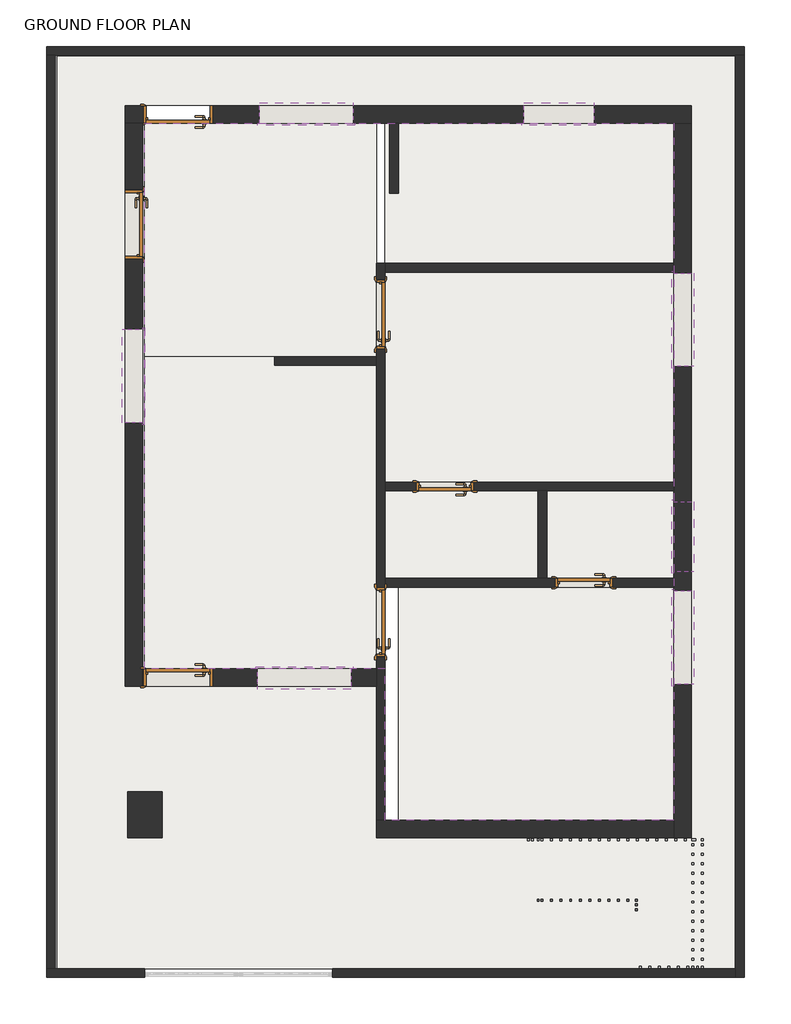
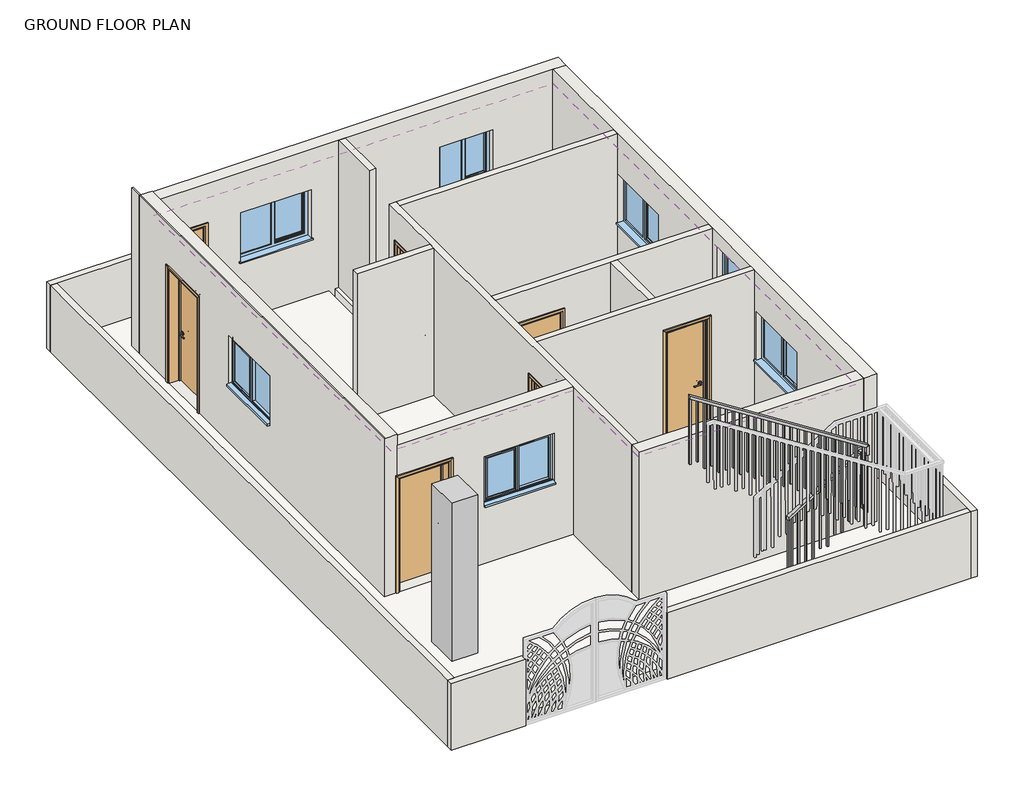
# One storey, part 1 of 23: 17 walls, 8 slabs, 7 doors, 7 windows, 1 column, 1 covering, 1 railing.
"""IFC4 building model written with IfcOpenShell, lengths in millimetres."""

from ifc_helpers import new_model, si_unit, frame, origin, place, context, project, spatial, polyline, outline, extrude, faceted_brep, transform, mapped, element, save
from components import columns_rectangular_450x600mm_2bb2af66, doors_intsgl_d1_d2de26da, doors_intsgl_d1_5aeab8eb, doors_intsgl_d1_91024936, doors_intsgl_d2_21b53886, doors_intsgl_d2_1f5f3f16, windows_dbl_plain_w1_9e0d93ab, windows_dbl_plain_w2_c69f14ef, windows_sgl_plain_v_28d0678b

model = new_model("IFC4")

# Units and contexts
model_context = context("Model", 3, world=origin())
ifc_project = project(units=[si_unit("LENGTHUNIT", "METRE", prefix="MILLI")], contexts=[model_context])

# Site, building, storey
site = spatial("IfcSite", under=ifc_project)
building = spatial("IfcBuilding", under=site)
storey = spatial("IfcBuildingStorey", under=building, Name="GROUND FLOOR PLAN", Elevation=487.68)

# Column
placement = place(None, origin())
columns_rectangular_450x600mm_shape = columns_rectangular_450x600mm_2bb2af66(model_context)
element("IfcColumn", 1, ObjectType="Columns_Rectangular : 450x600mm", at=placement, inside=storey, context=model_context, shape_type="MappedRepresentation", body=[
    mapped(columns_rectangular_450x600mm_shape, transform((-13810.4335145, -9915.2345894, 0.0), x_axis=(0.0, 1.0, 0.0), y_axis=(-1.0, 0.0, 0.0), z_axis=(0.0, 0.0, 1.0))),
])

# Covering
element("IfcCovering", 2, at=placement, inside=storey, context=model_context, shape_type="SweptSolid", body=[
    extrude(outline(polyline([(-6897.0620435, -885.5593981), (-6897.0620435, -9991.0521308), (-10668.9827978, -9991.0521308), (-10668.9827978, -8010.2345894), (-13810.6009005, -8010.2345894), (-13810.6009005, -885.5593981), (-6897.0620435, -885.5593981)])), frame((0.0, 0.0, 3078.48), z_axis=(0.0, 0.0, 1.0), x_axis=(1.0, 0.0, 0.0)), (0.0, 0.0, 1.0), 57.0),
])

# Doors
doors_intsgl_d1_shape = doors_intsgl_d1_d2de26da(model_context)
element("IfcDoor", 3, ObjectType="Doors_IntSgl : D1", at=placement, inside=storey, context=model_context, shape_type="MappedRepresentation", body=[
    mapped(doors_intsgl_d1_shape, transform((-10726.1327978, -7400.866169, 637.6416), x_axis=(0.0, 1.0, 0.0), y_axis=(-1.0, 0.0, 0.0), z_axis=(0.0, 0.0, 1.0))),
])
element("IfcDoor", 4, ObjectType="Doors_IntSgl : D1", at=placement, inside=storey, context=model_context, shape_type="MappedRepresentation", body=[
    mapped(doors_intsgl_d1_shape, transform((-10726.1327978, -3381.2262014, 637.6416), x_axis=(0.0, 1.0, 0.0), y_axis=(-1.0, 0.0, 0.0), z_axis=(0.0, 0.0, 1.0))),
])
doors_intsgl_d1_2_shape = doors_intsgl_d1_5aeab8eb(model_context)
element("IfcDoor", 5, ObjectType="Doors_IntSgl : D1", at=placement, inside=storey, context=model_context, shape_type="MappedRepresentation", body=[
    mapped(doors_intsgl_d1_2_shape, transform((-13373.8823015, -8124.5345894, 637.6416), x_axis=(-1.0, 0.0, 0.0), y_axis=(0.0, -1.0, 0.0), z_axis=(0.0, 0.0, 1.0))),
])
doors_intsgl_d1_3_shape = doors_intsgl_d1_91024936(model_context)
element("IfcDoor", 6, ObjectType="Doors_IntSgl : D1", at=placement, inside=storey, context=model_context, shape_type="MappedRepresentation", body=[
    mapped(doors_intsgl_d1_3_shape, transform((-13950.6420435, -2206.3593981, 637.6416), x_axis=(0.0, -1.0, 0.0), y_axis=(1.0, 0.0, 0.0), z_axis=(0.0, 0.0, 1.0))),
])
element("IfcDoor", 7, ObjectType="Doors_IntSgl : D1", at=placement, inside=storey, context=model_context, shape_type="MappedRepresentation", body=[
    mapped(doors_intsgl_d1_3_shape, transform((-13373.8823015, -771.2593981, 487.68), x_axis=(-1.0, 0.0, 0.0), y_axis=(0.0, -1.0, 0.0), z_axis=(0.0, 0.0, 1.0))),
])
doors_intsgl_d2_shape = doors_intsgl_d2_21b53886(model_context)
element("IfcDoor", 8, ObjectType="Doors_IntSgl : D2", at=placement, inside=storey, context=model_context, shape_type="MappedRepresentation", body=[
    mapped(doors_intsgl_d2_shape, transform((-9886.3340108, -5628.9784114, 637.6416), x_axis=(-1.0, 0.0, 0.0), y_axis=(0.0, -1.0, 0.0), z_axis=(0.0, 0.0, 1.0))),
])
doors_intsgl_d2_2_shape = doors_intsgl_d2_1f5f3f16(model_context)
element("IfcDoor", 9, ObjectType="Doors_IntSgl : D2", at=placement, inside=storey, context=model_context, shape_type="MappedRepresentation", body=[
    mapped(doors_intsgl_d2_2_shape, transform((-8070.4366309, -6886.516169, 637.6416), x_axis=(-1.0, 0.0, 0.0), y_axis=(0.0, -1.0, 0.0), z_axis=(0.0, 0.0, 1.0))),
])

# Railing
element("IfcRailing", 10, ObjectType="1100mm", at=placement, inside=storey, context=model_context, shape_type="SolidModel", body=[
    faceted_brep([(-8680.149573, -11007.9255223, 1912.8), (-8680.149573, -11007.9255223, 1853.4423995), (-8680.149573, -11057.9255223, 1853.4423995), (-8680.149573, -11057.9255223, 1912.8), (-7484.3306254, -11007.9255223, 2677.8717446), (-7434.3306254, -11007.9255223, 2650.5035914), (-7434.3306254, -11057.9255223, 2650.5035914), (-7484.3306254, -11057.9255223, 2677.8717446), (-7484.3306254, -11007.9255223, 2725.6), (-7434.3306254, -11007.9255223, 2675.6), (-7434.3306254, -11057.9255223, 2675.6), (-7484.3306254, -11057.9255223, 2725.6), (-7359.3306254, -11007.9255223, 2725.6), (-7359.3306254, -11007.9255223, 2675.6), (-7409.3306254, -11057.9255223, 2675.6), (-7409.3306254, -11057.9255223, 2725.6), (-7359.3306254, -11132.9255223, 2725.6), (-7359.3306254, -11132.9255223, 2675.6), (-7409.3306254, -11132.9255223, 2675.6), (-7409.3306254, -11132.9255223, 2725.6), (-7359.3306254, -11134.9255223, 2725.6), (-7409.3306254, -11134.9255223, 2725.6), (-7409.3306254, -11184.9255223, 2675.6), (-7359.3306254, -11184.9255223, 2675.6)], [[[0, 1, 2, 3]], [[1, 0, 4, 5]], [[2, 1, 5, 6]], [[3, 2, 6, 7]], [[0, 3, 7, 4]], [[5, 4, 8, 9]], [[6, 5, 9, 10]], [[7, 6, 10, 11]], [[4, 7, 11, 8]], [[9, 8, 12, 13]], [[10, 9, 13, 14]], [[11, 10, 14, 15]], [[8, 11, 15, 12]], [[13, 12, 16, 17]], [[14, 13, 17, 18]], [[15, 14, 18, 19]], [[12, 15, 19, 16]], [[20, 21, 22, 23]], [[17, 16, 20, 23]], [[18, 17, 23, 22]], [[19, 18, 22, 21]], [[16, 19, 21, 20]]]),
    faceted_brep([(-7359.3306254, -11134.9255223, 2725.6), (-7359.3306254, -11184.9255223, 2675.6), (-7409.3306254, -11184.9255223, 2675.6), (-7409.3306254, -11134.9255223, 2725.6), (-7359.3306254, -11134.9255223, 2855.9055527), (-7409.3306254, -11134.9255223, 2828.5415543), (-7409.3306254, -11184.9255223, 2828.5415543), (-7359.3306254, -11184.9255223, 2855.9055527)], [[[0, 1, 2, 3]], [[4, 5, 6, 7]], [[1, 0, 4, 7]], [[2, 1, 7, 6]], [[3, 2, 6, 5]], [[0, 3, 5, 4]]]),
    faceted_brep([(-7359.3306254, -11184.9255223, 2855.9055527), (-7409.3306254, -11184.9255223, 2828.5415543), (-7409.3306254, -11134.9255223, 2828.5415543), (-7359.3306254, -11134.9255223, 2855.9055527), (-10457.8773536, -11184.9255223, 4838.88), (-10457.8773536, -11134.9255223, 4838.88), (-10457.8773536, -11134.9255223, 4779.517542), (-10457.8773536, -11184.9255223, 4779.517542)], [[[0, 1, 2, 3]], [[4, 5, 6, 7]], [[1, 0, 4, 7]], [[2, 1, 7, 6]], [[3, 2, 6, 5]], [[0, 3, 5, 4]]]),
    extrude(outline(polyline([(3576.32, -10434.3306254), (4764.4483614, -10434.3306254), (4780.4475912, -10459.3306254), (3576.32, -10459.3306254), (3576.32, -10434.3306254)])), frame((0.0, -11172.4255223, 0.0), z_axis=(0.0, 1.0, 0.0), x_axis=(0.0, 0.0, 1.0)), (0.0, 0.0, 1.0), 25.0),
    extrude(outline(polyline([(3576.32, -10309.3306254), (4684.4522123, -10309.3306254), (4700.4514422, -10334.3306254), (3576.32, -10334.3306254), (3576.32, -10309.3306254)])), frame((0.0, -11172.4255223, 0.0), z_axis=(0.0, 1.0, 0.0), x_axis=(0.0, 0.0, 1.0)), (0.0, 0.0, 1.0), 25.0),
    extrude(outline(polyline([(3413.76, -10184.3306254), (4604.4560633, -10184.3306254), (4620.4552931, -10209.3306254), (3413.76, -10209.3306254), (3413.76, -10184.3306254)])), frame((0.0, -11172.4255223, 0.0), z_axis=(0.0, 1.0, 0.0), x_axis=(0.0, 0.0, 1.0)), (0.0, 0.0, 1.0), 25.0),
    extrude(outline(polyline([(3413.76, -10059.3306254), (4524.4599142, -10059.3306254), (4540.459144, -10084.3306254), (3413.76, -10084.3306254), (3413.76, -10059.3306254)])), frame((0.0, -11172.4255223, 0.0), z_axis=(0.0, 1.0, 0.0), x_axis=(0.0, 0.0, 1.0)), (0.0, 0.0, 1.0), 25.0),
    extrude(outline(polyline([(3251.2, -9934.3306254), (4444.4637652, -9934.3306254), (4460.462995, -9959.3306254), (3251.2, -9959.3306254), (3251.2, -9934.3306254)])), frame((0.0, -11172.4255223, 0.0), z_axis=(0.0, 1.0, 0.0), x_axis=(0.0, 0.0, 1.0)), (0.0, 0.0, 1.0), 25.0),
    extrude(outline(polyline([(3251.2, -9809.3306254), (4364.4676161, -9809.3306254), (4380.4668459, -9834.3306254), (3251.2, -9834.3306254), (3251.2, -9809.3306254)])), frame((0.0, -11172.4255223, 0.0), z_axis=(0.0, 1.0, 0.0), x_axis=(0.0, 0.0, 1.0)), (0.0, 0.0, 1.0), 25.0),
    extrude(outline(polyline([(3251.2, -9684.3306254), (4284.4714671, -9684.3306254), (4300.4706969, -9709.3306254), (3251.2, -9709.3306254), (3251.2, -9684.3306254)])), frame((0.0, -11172.4255223, 0.0), z_axis=(0.0, 1.0, 0.0), x_axis=(0.0, 0.0, 1.0)), (0.0, 0.0, 1.0), 25.0),
    extrude(outline(polyline([(3088.64, -9559.3306254), (4204.475318, -9559.3306254), (4220.4745478, -9584.3306254), (3088.64, -9584.3306254), (3088.64, -9559.3306254)])), frame((0.0, -11172.4255223, 0.0), z_axis=(0.0, 1.0, 0.0), x_axis=(0.0, 0.0, 1.0)), (0.0, 0.0, 1.0), 25.0),
    extrude(outline(polyline([(3088.64, -9434.3306254), (4124.479169, -9434.3306254), (4140.4783988, -9459.3306254), (3088.64, -9459.3306254), (3088.64, -9434.3306254)])), frame((0.0, -11172.4255223, 0.0), z_axis=(0.0, 1.0, 0.0), x_axis=(0.0, 0.0, 1.0)), (0.0, 0.0, 1.0), 25.0),
    extrude(outline(polyline([(2926.08, -9309.3306254), (4044.4830199, -9309.3306254), (4060.4822497, -9334.3306254), (2926.08, -9334.3306254), (2926.08, -9309.3306254)])), frame((0.0, -11172.4255223, 0.0), z_axis=(0.0, 1.0, 0.0), x_axis=(0.0, 0.0, 1.0)), (0.0, 0.0, 1.0), 25.0),
    extrude(outline(polyline([(2926.08, -9184.3306254), (3964.4868709, -9184.3306254), (3980.4861007, -9209.3306254), (2926.08, -9209.3306254), (2926.08, -9184.3306254)])), frame((0.0, -11172.4255223, 0.0), z_axis=(0.0, 1.0, 0.0), x_axis=(0.0, 0.0, 1.0)), (0.0, 0.0, 1.0), 25.0),
    extrude(outline(polyline([(2763.52, -9059.3306254), (3884.4907218, -9059.3306254), (3900.4899516, -9084.3306254), (2763.52, -9084.3306254), (2763.52, -9059.3306254)])), frame((0.0, -11172.4255223, 0.0), z_axis=(0.0, 1.0, 0.0), x_axis=(0.0, 0.0, 1.0)), (0.0, 0.0, 1.0), 25.0),
    extrude(outline(polyline([(2763.52, -8934.3306254), (3804.4945728, -8934.3306254), (3820.4938026, -8959.3306254), (2763.52, -8959.3306254), (2763.52, -8934.3306254)])), frame((0.0, -11172.4255223, 0.0), z_axis=(0.0, 1.0, 0.0), x_axis=(0.0, 0.0, 1.0)), (0.0, 0.0, 1.0), 25.0),
    extrude(outline(polyline([(2600.96, -8809.3306254), (3724.4984237, -8809.3306254), (3740.4976535, -8834.3306254), (2600.96, -8834.3306254), (2600.96, -8809.3306254)])), frame((0.0, -11172.4255223, 0.0), z_axis=(0.0, 1.0, 0.0), x_axis=(0.0, 0.0, 1.0)), (0.0, 0.0, 1.0), 25.0),
    extrude(outline(polyline([(2600.96, -8684.3306254), (3644.5022747, -8684.3306254), (3660.5015045, -8709.3306254), (2600.96, -8709.3306254), (2600.96, -8684.3306254)])), frame((0.0, -11172.4255223, 0.0), z_axis=(0.0, 1.0, 0.0), x_axis=(0.0, 0.0, 1.0)), (0.0, 0.0, 1.0), 25.0),
    extrude(outline(polyline([(2438.4, -8559.3306254), (3564.5061256, -8559.3306254), (3580.5053554, -8584.3306254), (2438.4, -8584.3306254), (2438.4, -8559.3306254)])), frame((0.0, -11172.4255223, 0.0), z_axis=(0.0, 1.0, 0.0), x_axis=(0.0, 0.0, 1.0)), (0.0, 0.0, 1.0), 25.0),
    extrude(outline(polyline([(2438.4, -8434.3306254), (3484.5099766, -8434.3306254), (3500.5092064, -8459.3306254), (2438.4, -8459.3306254), (2438.4, -8434.3306254)])), frame((0.0, -11172.4255223, 0.0), z_axis=(0.0, 1.0, 0.0), x_axis=(0.0, 0.0, 1.0)), (0.0, 0.0, 1.0), 25.0),
    extrude(outline(polyline([(2275.84, -8309.3306254), (3404.5138275, -8309.3306254), (3420.5130573, -8334.3306254), (2275.84, -8334.3306254), (2275.84, -8309.3306254)])), frame((0.0, -11172.4255223, 0.0), z_axis=(0.0, 1.0, 0.0), x_axis=(0.0, 0.0, 1.0)), (0.0, 0.0, 1.0), 25.0),
    extrude(outline(polyline([(2275.84, -8184.3306254), (3324.5176785, -8184.3306254), (3340.5169083, -8209.3306254), (2275.84, -8209.3306254), (2275.84, -8184.3306254)])), frame((0.0, -11172.4255223, 0.0), z_axis=(0.0, 1.0, 0.0), x_axis=(0.0, 0.0, 1.0)), (0.0, 0.0, 1.0), 25.0),
    extrude(outline(polyline([(2113.28, -8059.3306254), (3244.5215294, -8059.3306254), (3260.5207592, -8084.3306254), (2113.28, -8084.3306254), (2113.28, -8059.3306254)])), frame((0.0, -11172.4255223, 0.0), z_axis=(0.0, 1.0, 0.0), x_axis=(0.0, 0.0, 1.0)), (0.0, 0.0, 1.0), 25.0),
    extrude(outline(polyline([(2113.28, -7934.3306254), (3164.5253804, -7934.3306254), (3180.5246102, -7959.3306254), (2113.28, -7959.3306254), (2113.28, -7934.3306254)])), frame((0.0, -11172.4255223, 0.0), z_axis=(0.0, 1.0, 0.0), x_axis=(0.0, 0.0, 1.0)), (0.0, 0.0, 1.0), 25.0),
    extrude(outline(polyline([(1950.72, -7809.3306254), (3084.5292313, -7809.3306254), (3100.5284611, -7834.3306254), (1950.72, -7834.3306254), (1950.72, -7809.3306254)])), frame((0.0, -11172.4255223, 0.0), z_axis=(0.0, 1.0, 0.0), x_axis=(0.0, 0.0, 1.0)), (0.0, 0.0, 1.0), 25.0),
    extrude(outline(polyline([(1950.72, -7684.3306254), (3004.5330823, -7684.3306254), (3020.5323121, -7709.3306254), (1950.72, -7709.3306254), (1950.72, -7684.3306254)])), frame((0.0, -11172.4255223, 0.0), z_axis=(0.0, 1.0, 0.0), x_axis=(0.0, 0.0, 1.0)), (0.0, 0.0, 1.0), 25.0),
    extrude(outline(polyline([(1788.16, -7559.3306254), (2924.5369332, -7559.3306254), (2940.536163, -7584.3306254), (1788.16, -7584.3306254), (1788.16, -7559.3306254)])), frame((0.0, -11172.4255223, 0.0), z_axis=(0.0, 1.0, 0.0), x_axis=(0.0, 0.0, 1.0)), (0.0, 0.0, 1.0), 25.0),
    extrude(outline(polyline([(1788.16, -7434.3306254), (2844.5407841, -7434.3306254), (2860.540014, -7459.3306254), (1788.16, -7459.3306254), (1788.16, -7434.3306254)])), frame((0.0, -11172.4255223, 0.0), z_axis=(0.0, 1.0, 0.0), x_axis=(0.0, 0.0, 1.0)), (0.0, 0.0, 1.0), 25.0),
    extrude(outline(polyline([(-7396.8306254, -11082.9255223), (-7371.8306254, -11082.9255223), (-7371.8306254, -11107.9255223), (-7396.8306254, -11107.9255223), (-7396.8306254, -11082.9255223)])), frame((0.0, 0.0, 1625.6), z_axis=(0.0, 0.0, 1.0), x_axis=(1.0, 0.0, 0.0)), (0.0, 0.0, 1.0), 1050.0),
    extrude(outline(polyline([(2605.1944115, -7505.149573), (1463.04, -7505.149573), (1463.04, -7480.149573), (2621.1891352, -7480.149573), (2605.1944115, -7505.149573)])), frame((0.0, -11045.4255223, 0.0), z_axis=(0.0, 1.0, 0.0), x_axis=(0.0, 0.0, 1.0)), (0.0, 0.0, 1.0), 25.0),
    extrude(outline(polyline([(2525.2207932, -7630.149573), (1463.04, -7630.149573), (1463.04, -7605.149573), (2541.2155169, -7605.149573), (2525.2207932, -7630.149573)])), frame((0.0, -11045.4255223, 0.0), z_axis=(0.0, 1.0, 0.0), x_axis=(0.0, 0.0, 1.0)), (0.0, 0.0, 1.0), 25.0),
    extrude(outline(polyline([(2445.2471749, -7755.149573), (1300.48, -7755.149573), (1300.48, -7730.149573), (2461.2418986, -7730.149573), (2445.2471749, -7755.149573)])), frame((0.0, -11045.4255223, 0.0), z_axis=(0.0, 1.0, 0.0), x_axis=(0.0, 0.0, 1.0)), (0.0, 0.0, 1.0), 25.0),
    extrude(outline(polyline([(2365.2735566, -7880.149573), (1300.48, -7880.149573), (1300.48, -7855.149573), (2381.2682803, -7855.149573), (2365.2735566, -7880.149573)])), frame((0.0, -11045.4255223, 0.0), z_axis=(0.0, 1.0, 0.0), x_axis=(0.0, 0.0, 1.0)), (0.0, 0.0, 1.0), 25.0),
    extrude(outline(polyline([(2285.2999383, -8005.149573), (1137.92, -8005.149573), (1137.92, -7980.149573), (2301.294662, -7980.149573), (2285.2999383, -8005.149573)])), frame((0.0, -11045.4255223, 0.0), z_axis=(0.0, 1.0, 0.0), x_axis=(0.0, 0.0, 1.0)), (0.0, 0.0, 1.0), 25.0),
    extrude(outline(polyline([(2205.32632, -8130.149573), (1137.92, -8130.149573), (1137.92, -8105.149573), (2221.3210437, -8105.149573), (2205.32632, -8130.149573)])), frame((0.0, -11045.4255223, 0.0), z_axis=(0.0, 1.0, 0.0), x_axis=(0.0, 0.0, 1.0)), (0.0, 0.0, 1.0), 25.0),
    extrude(outline(polyline([(2125.3527017, -8255.149573), (975.36, -8255.149573), (975.36, -8230.149573), (2141.3474254, -8230.149573), (2125.3527017, -8255.149573)])), frame((0.0, -11045.4255223, 0.0), z_axis=(0.0, 1.0, 0.0), x_axis=(0.0, 0.0, 1.0)), (0.0, 0.0, 1.0), 25.0),
    extrude(outline(polyline([(2045.3790834, -8380.149573), (975.36, -8380.149573), (975.36, -8355.149573), (2061.3738071, -8355.149573), (2045.3790834, -8380.149573)])), frame((0.0, -11045.4255223, 0.0), z_axis=(0.0, 1.0, 0.0), x_axis=(0.0, 0.0, 1.0)), (0.0, 0.0, 1.0), 25.0),
    extrude(outline(polyline([(1965.4054651, -8505.149573), (812.8, -8505.149573), (812.8, -8480.149573), (1981.4001888, -8480.149573), (1965.4054651, -8505.149573)])), frame((0.0, -11045.4255223, 0.0), z_axis=(0.0, 1.0, 0.0), x_axis=(0.0, 0.0, 1.0)), (0.0, 0.0, 1.0), 25.0),
    extrude(outline(polyline([(1885.4318468, -8630.149573), (812.8, -8630.149573), (812.8, -8605.149573), (1901.4265705, -8605.149573), (1885.4318468, -8630.149573)])), frame((0.0, -11045.4255223, 0.0), z_axis=(0.0, 1.0, 0.0), x_axis=(0.0, 0.0, 1.0)), (0.0, 0.0, 1.0), 25.0),
    extrude(outline(polyline([(-7396.8306254, -11147.4255223), (-7371.8306254, -11147.4255223), (-7371.8306254, -11172.4255223), (-7396.8306254, -11172.4255223), (-7396.8306254, -11147.4255223)])), frame((0.0, 0.0, 1625.6), z_axis=(0.0, 0.0, 1.0), x_axis=(1.0, 0.0, 0.0)), (0.0, 0.0, 1.0), 1050.0),
    extrude(outline(polyline([(-7396.8306254, -11045.4255223), (-7396.8306254, -11020.4255223), (-7371.8306254, -11020.4255223), (-7371.8306254, -11045.4255223), (-7396.8306254, -11045.4255223)])), frame((0.0, 0.0, 1625.6), z_axis=(0.0, 0.0, 1.0), x_axis=(1.0, 0.0, 0.0)), (0.0, 0.0, 1.0), 1050.0),
    extrude(outline(polyline([(3576.32, -10432.8773536), (4763.5183122, -10432.8773536), (4779.517542, -10457.8773536), (3576.32, -10457.8773536), (3576.32, -10432.8773536)])), frame((0.0, -11172.4255223, 0.0), z_axis=(0.0, 1.0, 0.0), x_axis=(0.0, 0.0, 1.0)), (0.0, 0.0, 1.0), 25.0),
    extrude(outline(polyline([(1853.4423995, -8680.149573), (812.8, -8680.149573), (812.8, -8655.149573), (1869.4371231, -8655.149573), (1853.4423995, -8680.149573)])), frame((0.0, -11045.4255223, 0.0), z_axis=(0.0, 1.0, 0.0), x_axis=(0.0, 0.0, 1.0)), (0.0, 0.0, 1.0), 25.0),
])

# Slabs
element("IfcSlab", 11, ObjectType="BATHROOM FLOORING", at=placement, inside=storey, context=model_context, shape_type="SweptSolid", body=[
    extrude(outline(polyline([(-8667.3366309, -5686.1284114), (-8667.3366309, -6829.366169), (-10668.9827978, -6829.366169), (-10668.9827978, -5686.1284114), (-8667.3366309, -5686.1284114)])), frame((0.0, 0.0, 487.68), z_axis=(0.0, 0.0, 1.0), x_axis=(1.0, 0.0, 0.0)), (0.0, 0.0, 1.0), 149.9616),
])
element("IfcSlab", 12, ObjectType="BATHROOM FLOORING", at=placement, inside=storey, context=model_context, shape_type="SweptSolid", body=[
    extrude(outline(polyline([(-6724.371003, -5686.0601635), (-6724.371003, -6829.366169), (-8553.0366309, -6829.366169), (-8553.0366309, -5686.0601635), (-6724.371003, -5686.0601635)])), frame((0.0, 0.0, 487.68), z_axis=(0.0, 0.0, 1.0), x_axis=(1.0, 0.0, 0.0)), (0.0, 0.0, 1.0), 149.9616),
])
element("IfcSlab", 13, ObjectType="BED ROOM FLOORING", at=placement, inside=storey, context=model_context, shape_type="SweptSolid", body=[
    extrude(outline(polyline([(-6724.371003, -2828.9136626), (-6724.371003, -5571.8284114), (-10668.9827978, -5571.8284114), (-10668.9827978, -2828.9136626), (-6724.371003, -2828.9136626)])), frame((0.0, 0.0, 487.68), z_axis=(0.0, 0.0, 1.0), x_axis=(1.0, 0.0, 0.0)), (0.0, 0.0, 1.0), 149.9616),
])
element("IfcSlab", 14, ObjectType="BED ROOM FLOORING", at=placement, inside=storey, context=model_context, shape_type="SweptSolid", body=[
    extrude(outline(polyline([(-6698.6395131, -6943.5979211), (-6698.6395131, -9991.1886267), (-10495.9340108, -9991.1886267), (-10495.9340108, -6943.5979211), (-6698.6395131, -6943.5979211)])), frame((0.0, 0.0, 487.68), z_axis=(0.0, 0.0, 1.0), x_axis=(1.0, 0.0, 0.0)), (0.0, 0.0, 1.0), 149.9616),
])
element("IfcSlab", 15, ObjectType="DINING FLOORING", at=placement, inside=storey, context=model_context, shape_type="SweptSolid", body=[
    extrude(outline(polyline([(-10783.2827978, -885.9480347), (-10783.2827978, -3933.5387403), (-13810.6009005, -3933.5387403), (-13810.6009005, -885.9480347), (-10783.2827978, -885.9480347)])), frame((0.0, 0.0, 487.68), z_axis=(0.0, 0.0, 1.0), x_axis=(1.0, 0.0, 0.0)), (0.0, 0.0, 1.0), 149.9616),
])
element("IfcSlab", 16, ObjectType="HALL FLOORING", at=placement, inside=storey, context=model_context, shape_type="SweptSolid", body=[
    extrude(outline(polyline([(-10783.2827978, -3933.5387403), (-10783.2827978, -8010.2345894), (-13810.6009005, -8010.2345894), (-13810.6009005, -3933.5387403), (-10783.2827978, -3933.5387403)])), frame((0.0, 0.0, 487.68), z_axis=(0.0, 0.0, 1.0), x_axis=(1.0, 0.0, 0.0)), (0.0, 0.0, 1.0), 149.9616),
])
element("IfcSlab", 17, ObjectType="KITCHEN FLOOR", at=placement, inside=storey, context=model_context, shape_type="SweptSolid", body=[
    extrude(outline(polyline([(-6724.371003, -885.9480347), (-6724.371003, -2714.6136626), (-10668.9827978, -2714.6136626), (-10668.9827978, -885.9480347), (-6724.371003, -885.9480347)])), frame((0.0, 0.0, 487.68), z_axis=(0.0, 0.0, 1.0), x_axis=(1.0, 0.0, 0.0)), (0.0, 0.0, 1.0), 149.9616),
])
element("IfcSlab", 18, ObjectType="OUTER FLOORING", at=placement, inside=storey, context=model_context, shape_type="Brep", body=[
    faceted_brep([(-6089.3420435, -9.6873231, 487.68), (-6089.3420435, -11928.1928911, 487.68), (-14953.3817735, -11928.1928911, 487.68), (-14953.3817735, -9.6873231, 487.68), (-6668.4620435, -656.9593981, 487.68), (-12916.6823015, -656.9593981, 487.68), (-13831.0823015, -656.9593981, 487.68), (-14064.9420435, -656.9593981, 487.68), (-14064.9420435, -885.5593981, 487.68), (-14064.9420435, -8238.8345894, 487.68), (-13836.3420435, -8238.8345894, 487.68), (-10783.2827978, -8238.8345894, 487.68), (-10783.2827978, -9991.0521308, 487.68), (-10783.2827978, -10219.6521308, 487.68), (-6897.0620435, -10219.6521308, 487.68), (-6668.4620435, -10219.6521308, 487.68), (-6668.4620435, -885.5593981, 487.68), (-6089.3420435, -9.6873231, 637.6416), (-14953.3817735, -9.6873231, 637.6416), (-14953.3817735, -11928.1928911, 637.6416), (-6089.3420435, -11928.1928911, 637.6416), (-6668.4620435, -656.9593981, 637.6416), (-6668.4620435, -10219.6521308, 637.6416), (-10783.2827978, -10219.6521308, 637.6416), (-10783.2827978, -8238.8345894, 637.6416), (-12916.6823015, -8238.8345894, 637.6416), (-13831.0823015, -8238.8345894, 637.6416), (-14064.9420435, -8238.8345894, 637.6416), (-14064.9420435, -2663.5593981, 637.6416), (-14064.9420435, -1749.1593981, 637.6416), (-14064.9420435, -656.9593981, 637.6416)], [[[0, 1, 2, 3], [4, 5, 6, 7, 8, 9, 10, 11, 12, 13, 14, 15, 16]], [[17, 18, 19, 20], [21, 22, 23, 24, 25, 26, 27, 28, 29, 30]], [[1, 0, 17, 20]], [[2, 1, 20, 19]], [[3, 2, 19, 18]], [[0, 3, 18, 17]], [[7, 6, 5, 4, 21, 30]], [[9, 8, 7, 30, 29, 28, 27]], [[11, 10, 9, 27, 26, 25, 24]], [[13, 12, 11, 24, 23]], [[15, 14, 13, 23, 22]], [[4, 16, 15, 22, 21]]]),
])

# Walls
element("IfcWall", 19, at=placement, inside=storey, context=model_context, shape_type="Brep", body=[
    faceted_brep([(-15093.6420435, 3.4571089, 487.68), (-14979.3420435, 3.4571089, 487.68), (-6089.3420435, 3.4571089, 487.68), (-5975.0420435, 3.4571089, 487.68), (-5975.0420435, 3.4571089, 1706.88), (-6089.3420435, 3.4571089, 1706.88), (-14979.3420435, 3.4571089, 1706.88), (-15093.6420435, 3.4571089, 1706.88), (-15093.6420435, 117.7571089, 487.68), (-15093.6420435, 117.7571089, 1706.88), (-5975.0420435, 117.7571089, 1706.88), (-5975.0420435, 117.7571089, 487.68)], [[[0, 1, 2, 3, 4, 5, 6, 7]], [[8, 9, 10, 11]], [[3, 2, 1, 0, 8, 11]], [[7, 6, 5, 4, 10, 9]], [[4, 3, 11, 10]], [[0, 7, 9, 8]]]),
])
element("IfcWall", 20, at=placement, inside=storey, context=model_context, shape_type="Brep", body=[
    faceted_brep([(-6089.3420435, 3.4571089, 487.68), (-6089.3420435, -11928.1928911, 487.68), (-6089.3420435, -12042.4928911, 487.68), (-6089.3420435, -12042.4928911, 1706.88), (-6089.3420435, -11928.1928911, 1706.88), (-6089.3420435, 3.4571089, 1706.88), (-5975.0420435, 3.4571089, 487.68), (-5975.0420435, 3.4571089, 1706.88), (-5975.0420435, -12042.4928911, 1706.88), (-5975.0420435, -12042.4928911, 487.68)], [[[0, 1, 2, 3, 4, 5]], [[6, 7, 8, 9]], [[2, 1, 0, 6, 9]], [[5, 4, 3, 8, 7]], [[0, 5, 7, 6]], [[3, 2, 9, 8]]]),
])
element("IfcWall", 21, at=placement, inside=storey, context=model_context, shape_type="SweptSolid", body=[
    extrude(outline(polyline([(-11356.3590108, -11928.1928911), (-6089.3420435, -11928.1928911), (-6089.3420435, -12042.4928911), (-11356.3590108, -12042.4928911), (-11356.3590108, -11928.1928911)])), frame((0.0, 0.0, 487.68), z_axis=(0.0, 0.0, 1.0), x_axis=(1.0, 0.0, 0.0)), (0.0, 0.0, 1.0), 1219.2),
])
element("IfcWall", 22, at=placement, inside=storey, context=model_context, shape_type="SweptSolid", body=[
    extrude(outline(polyline([(-14979.3420435, 3.4571089), (-14979.3420435, -11928.1928911), (-15093.6420435, -11928.1928911), (-15093.6420435, 3.4571089), (-14979.3420435, 3.4571089)])), frame((0.0, 0.0, 487.68), z_axis=(0.0, 0.0, 1.0), x_axis=(1.0, 0.0, 0.0)), (0.0, 0.0, 1.0), 1219.2),
])
element("IfcWall", 23, at=placement, inside=storey, context=model_context, shape_type="Brep", body=[
    faceted_brep([(-13810.4335145, -11928.1928911, 487.68), (-14979.3420435, -11928.1928911, 487.68), (-15093.6420435, -11928.1928911, 487.68), (-15093.6420435, -11928.1928911, 1706.88), (-14979.3420435, -11928.1928911, 1706.88), (-13810.4335145, -11928.1928911, 1706.88), (-13810.4335145, -12042.4928911, 487.68), (-13810.4335145, -12042.4928911, 1706.88), (-15093.6420435, -12042.4928911, 1706.88), (-15093.6420435, -12042.4928911, 487.68)], [[[0, 1, 2, 3, 4, 5]], [[6, 7, 8, 9]], [[2, 1, 0, 6, 9]], [[5, 4, 3, 8, 7]], [[0, 5, 7, 6]], [[3, 2, 9, 8]]]),
])
element("IfcWall", 24, ObjectType="EXT WALL", at=placement, inside=storey, context=model_context, shape_type="Brep", body=[
    faceted_brep([(-14064.9420435, -885.5593981, 487.68), (-13836.3420435, -885.5593981, 487.68), (-13831.0823015, -885.5593981, 487.68), (-13831.0823015, -885.5593981, 2597.68), (-12916.6823015, -885.5593981, 2597.68), (-12916.6823015, -885.5593981, 487.68), (-6897.0620435, -885.5593981, 487.68), (-6668.4620435, -885.5593981, 487.68), (-6668.4620435, -885.5593981, 637.6416), (-6668.4620435, -885.5593981, 3335.7312), (-6897.0620435, -885.5593981, 3335.7312), (-14039.0335145, -885.5593981, 3335.7312), (-14039.0335145, -885.5593981, 3535.68), (-14064.9420435, -885.5593981, 3535.68), (-14064.9420435, -885.5593981, 637.6416), (-12307.0823015, -885.5593981, 1687.68), (-12307.0823015, -885.5593981, 2597.68), (-11087.8823015, -885.5593981, 2597.68), (-11087.8823015, -885.5593981, 1687.68), (-8852.8620435, -885.5593981, 1687.68), (-8852.8620435, -885.5593981, 2597.68), (-7938.4620435, -885.5593981, 2597.68), (-7938.4620435, -885.5593981, 1687.68), (-13831.0823015, -656.9593981, 487.68), (-14064.9420435, -656.9593981, 487.68), (-14064.9420435, -656.9593981, 637.6416), (-14064.9420435, -656.9593981, 3535.68), (-14039.0335145, -656.9593981, 3535.68), (-14039.0335145, -656.9593981, 3335.7312), (-6668.4620435, -656.9593981, 3335.7312), (-6668.4620435, -656.9593981, 637.6416), (-6668.4620435, -656.9593981, 487.68), (-12916.6823015, -656.9593981, 487.68), (-12916.6823015, -656.9593981, 637.6416), (-12916.6823015, -656.9593981, 2597.68), (-13831.0823015, -656.9593981, 2597.68), (-13831.0823015, -656.9593981, 637.6416), (-12307.0823015, -656.9593981, 2597.68), (-12307.0823015, -656.9593981, 1687.68), (-11087.8823015, -656.9593981, 1687.68), (-11087.8823015, -656.9593981, 2597.68), (-8852.8620435, -656.9593981, 2597.68), (-8852.8620435, -656.9593981, 1687.68), (-7938.4620435, -656.9593981, 1687.68), (-7938.4620435, -656.9593981, 2597.68)], [[[0, 1, 2, 3, 4, 5, 6, 7, 8, 9, 10, 11, 12, 13, 14], [15, 16, 17, 18], [19, 20, 21, 22]], [[23, 24, 25, 26, 27, 28, 29, 30, 31, 32, 33, 34, 35, 36], [37, 38, 39, 40], [41, 42, 43, 44]], [[31, 7, 6, 5, 32]], [[0, 24, 23, 2, 1]], [[7, 31, 30, 29, 9, 8]], [[24, 0, 14, 13, 26, 25]], [[35, 3, 2, 23, 36]], [[3, 35, 34, 4]], [[4, 34, 33, 32, 5]], [[38, 37, 16, 15]], [[39, 38, 15, 18]], [[40, 39, 18, 17]], [[37, 40, 17, 16]], [[42, 41, 20, 19]], [[43, 42, 19, 22]], [[44, 43, 22, 21]], [[41, 44, 21, 20]], [[28, 11, 10, 9, 29]], [[11, 28, 27, 12]], [[13, 12, 27, 26]]]),
])
element("IfcWall", 25, ObjectType="EXT WALL", at=placement, inside=storey, context=model_context, shape_type="Brep", body=[
    faceted_brep([(-6897.0620435, -885.5593981, 487.68), (-6897.0620435, -5571.8284114, 487.68), (-6897.0620435, -5686.1284114, 487.68), (-6897.0620435, -9991.0521308, 487.68), (-6897.0620435, -10219.6521308, 487.68), (-6897.0620435, -10219.6521308, 637.6416), (-6897.0620435, -10219.6521308, 3335.7312), (-6897.0620435, -9991.0521308, 3335.7312), (-6897.0620435, -6943.666169, 3335.7312), (-6897.0620435, -6829.366169, 3335.7312), (-6897.0620435, -5686.1284114, 3335.7312), (-6897.0620435, -5571.8284114, 3335.7312), (-6897.0620435, -885.5593981, 3335.7312), (-6897.0620435, -6993.8521308, 1687.68), (-6897.0620435, -6993.8521308, 2597.68), (-6897.0620435, -8213.0521308, 2597.68), (-6897.0620435, -8213.0521308, 1687.68), (-6897.0620435, -2841.3593981, 1687.68), (-6897.0620435, -2841.3593981, 2597.68), (-6897.0620435, -4060.5593981, 2597.68), (-6897.0620435, -4060.5593981, 1687.68), (-6897.0620435, -5825.4521308, 2164.08), (-6897.0620435, -5825.4521308, 3074.08), (-6897.0620435, -6739.8521308, 3074.08), (-6897.0620435, -6739.8521308, 2164.08), (-6668.4620435, -10219.6521308, 487.68), (-6668.4620435, -885.5593981, 487.68), (-6668.4620435, -885.5593981, 637.6416), (-6668.4620435, -885.5593981, 3335.7312), (-6668.4620435, -10219.6521308, 3335.7312), (-6668.4620435, -10219.6521308, 637.6416), (-6668.4620435, -6993.8521308, 2597.68), (-6668.4620435, -6993.8521308, 1687.68), (-6668.4620435, -8213.0521308, 1687.68), (-6668.4620435, -8213.0521308, 2597.68), (-6668.4620435, -2841.3593981, 2597.68), (-6668.4620435, -2841.3593981, 1687.68), (-6668.4620435, -4060.5593981, 1687.68), (-6668.4620435, -4060.5593981, 2597.68), (-6668.4620435, -5825.4521308, 3074.08), (-6668.4620435, -5825.4521308, 2164.08), (-6668.4620435, -6739.8521308, 2164.08), (-6668.4620435, -6739.8521308, 3074.08)], [[[0, 1, 2, 3, 4, 5, 6, 7, 8, 9, 10, 11, 12], [13, 14, 15, 16], [17, 18, 19, 20], [21, 22, 23, 24]], [[25, 26, 27, 28, 29, 30], [31, 32, 33, 34], [35, 36, 37, 38], [39, 40, 41, 42]], [[4, 3, 2, 1, 0, 26, 25]], [[26, 0, 12, 28, 27]], [[4, 25, 30, 29, 6, 5]], [[32, 31, 14, 13]], [[33, 32, 13, 16]], [[34, 33, 16, 15]], [[31, 34, 15, 14]], [[36, 35, 18, 17]], [[37, 36, 17, 20]], [[38, 37, 20, 19]], [[35, 38, 19, 18]], [[40, 39, 22, 21]], [[41, 40, 21, 24]], [[42, 41, 24, 23]], [[39, 42, 23, 22]], [[12, 11, 10, 9, 8, 7, 6, 29, 28]]]),
])
element("IfcWall", 26, ObjectType="EXT WALL", at=placement, inside=storey, context=model_context, shape_type="Brep", body=[
    faceted_brep([(-6897.0620435, -9991.0521308, 487.68), (-10668.9827978, -9991.0521308, 487.68), (-10783.2827978, -9991.0521308, 487.68), (-10783.2827978, -9991.0521308, 637.6416), (-10783.2827978, -9991.0521308, 3335.7312), (-10668.9827978, -9991.0521308, 3335.7312), (-6897.0620435, -9991.0521308, 3335.7312), (-10783.2827978, -10219.6521308, 487.68), (-6897.0620435, -10219.6521308, 487.68), (-6897.0620435, -10219.6521308, 637.6416), (-6897.0620435, -10219.6521308, 3335.7312), (-10783.2827978, -10219.6521308, 3335.7312), (-10783.2827978, -10219.6521308, 637.6416)], [[[0, 1, 2, 3, 4, 5, 6]], [[7, 8, 9, 10, 11, 12]], [[2, 1, 0, 8, 7]], [[8, 0, 6, 10, 9]], [[2, 7, 12, 11, 4, 3]], [[6, 5, 4, 11, 10]]]),
])
element("IfcWall", 27, ObjectType="EXT WALL", at=placement, inside=storey, context=model_context, shape_type="Brep", body=[
    faceted_brep([(-14064.9420435, -885.5593981, 487.68), (-14064.9420435, -8238.8345894, 487.68), (-14064.9420435, -8238.8345894, 637.6416), (-14064.9420435, -8238.8345894, 3535.68), (-14064.9420435, -885.5593981, 3535.68), (-14064.9420435, -885.5593981, 637.6416), (-14064.9420435, -2663.5593981, 2747.6416), (-14064.9420435, -2663.5593981, 637.6416), (-14064.9420435, -1749.1593981, 637.6416), (-14064.9420435, -1749.1593981, 2747.6416), (-14064.9420435, -4797.1593981, 2597.68), (-14064.9420435, -4797.1593981, 1687.68), (-14064.9420435, -3577.9593981, 1687.68), (-14064.9420435, -3577.9593981, 2597.68), (-13836.3420435, -8238.8345894, 487.68), (-13836.3420435, -8010.2345894, 487.68), (-13836.3420435, -885.5593981, 487.68), (-13836.3420435, -885.5593981, 3535.68), (-13836.3420435, -8238.8345894, 3535.68), (-13836.3420435, -8238.8345894, 3335.7312), (-13836.3420435, -8238.8345894, 637.6416), (-13836.3420435, -2663.5593981, 637.6416), (-13836.3420435, -2663.5593981, 2747.6416), (-13836.3420435, -1749.1593981, 2747.6416), (-13836.3420435, -1749.1593981, 637.6416), (-13836.3420435, -4797.1593981, 1687.68), (-13836.3420435, -4797.1593981, 2597.68), (-13836.3420435, -3577.9593981, 2597.68), (-13836.3420435, -3577.9593981, 1687.68), (-14039.0335145, -885.5593981, 3535.68), (-14039.0335145, -8238.8345894, 3535.68)], [[[0, 1, 2, 3, 4, 5], [6, 7, 8, 9], [10, 11, 12, 13]], [[14, 15, 16, 17, 18, 19, 20], [21, 22, 23, 24], [25, 26, 27, 28]], [[1, 0, 16, 15, 14]], [[17, 16, 0, 5, 4, 29]], [[1, 14, 20, 19, 18, 30, 3, 2]], [[7, 6, 22, 21]], [[6, 9, 23, 22]], [[9, 8, 24, 23]], [[8, 7, 21, 24]], [[11, 10, 26, 25]], [[12, 11, 25, 28]], [[13, 12, 28, 27]], [[10, 13, 27, 26]], [[18, 17, 29, 30]], [[4, 3, 30, 29]]]),
])
element("IfcWall", 28, ObjectType="EXT WALL", at=placement, inside=storey, context=model_context, shape_type="Brep", body=[
    faceted_brep([(-13836.3420435, -8238.8345894, 487.68), (-10783.2827978, -8238.8345894, 487.68), (-10783.2827978, -8238.8345894, 637.6416), (-10783.2827978, -8238.8345894, 3335.7312), (-13836.3420435, -8238.8345894, 3335.7312), (-13836.3420435, -8238.8345894, 637.6416), (-13831.0823015, -8238.8345894, 637.6416), (-13831.0823015, -8238.8345894, 2747.6416), (-12916.6823015, -8238.8345894, 2747.6416), (-12916.6823015, -8238.8345894, 637.6416), (-11113.4827978, -8238.8345894, 2597.68), (-11113.4827978, -8238.8345894, 1687.68), (-12332.6827978, -8238.8345894, 1687.68), (-12332.6827978, -8238.8345894, 2597.68), (-10783.2827978, -8010.2345894, 487.68), (-13836.3420435, -8010.2345894, 487.68), (-13836.3420435, -8010.2345894, 3335.7312), (-10783.2827978, -8010.2345894, 3335.7312), (-13831.0823015, -8010.2345894, 2747.6416), (-13831.0823015, -8010.2345894, 637.6416), (-12916.6823015, -8010.2345894, 637.6416), (-12916.6823015, -8010.2345894, 2747.6416), (-11113.4827978, -8010.2345894, 1687.68), (-11113.4827978, -8010.2345894, 2597.68), (-12332.6827978, -8010.2345894, 2597.68), (-12332.6827978, -8010.2345894, 1687.68)], [[[0, 1, 2, 3, 4, 5], [6, 7, 8, 9], [10, 11, 12, 13]], [[14, 15, 16, 17], [18, 19, 20, 21], [22, 23, 24, 25]], [[1, 0, 15, 14]], [[15, 0, 5, 4, 16]], [[1, 14, 17, 3, 2]], [[18, 7, 6, 19]], [[7, 18, 21, 8]], [[8, 21, 20, 9]], [[19, 6, 9, 20]], [[11, 10, 23, 22]], [[12, 11, 22, 25]], [[13, 12, 25, 24]], [[10, 13, 24, 23]], [[4, 3, 17, 16]]]),
])
element("IfcWall", 29, ObjectType="INT WALL", at=placement, inside=storey, context=model_context, shape_type="SweptSolid", body=[
    extrude(outline(polyline([(-10610.2340108, -1800.3480347), (-10610.2340108, -885.9480347), (-10495.9340108, -885.9480347), (-10495.9340108, -1800.3480347), (-10610.2340108, -1800.3480347)])), frame((0.0, 0.0, 487.68), z_axis=(0.0, 0.0, 1.0), x_axis=(1.0, 0.0, 0.0)), (0.0, 0.0, 1.0), 2848.0512),
])
element("IfcWall", 30, ObjectType="INT WALL", at=placement, inside=storey, context=model_context, shape_type="SweptSolid", body=[
    extrude(outline(polyline([(-10668.9827978, -2714.6136626), (-6897.41979, -2714.6136626), (-6897.41979, -2828.9136626), (-10668.9827978, -2828.9136626), (-10668.9827978, -2714.6136626)])), frame((0.0, 0.0, 487.68), z_axis=(0.0, 0.0, 1.0), x_axis=(1.0, 0.0, 0.0)), (0.0, 0.0, 1.0), 2848.0512),
])
element("IfcWall", 31, ObjectType="INT WALL", at=placement, inside=storey, context=model_context, shape_type="Brep", body=[
    faceted_brep([(-10668.9827978, -5686.1284114, 487.68), (-8667.3366309, -5686.1284114, 487.68), (-8553.0366309, -5686.1284114, 487.68), (-6897.0620435, -5686.1284114, 487.68), (-6897.0620435, -5686.1284114, 3335.7312), (-8553.0366309, -5686.1284114, 3335.7312), (-8667.3366309, -5686.1284114, 3335.7312), (-10668.9827978, -5686.1284114, 3335.7312), (-10267.3340108, -5686.1284114, 637.6416), (-10267.3340108, -5686.1284114, 2747.6416), (-9505.3340108, -5686.1284114, 2747.6416), (-9505.3340108, -5686.1284114, 637.6416), (-6897.0620435, -5571.8284114, 487.68), (-10668.9827978, -5571.8284114, 487.68), (-10668.9827978, -5571.8284114, 3335.7312), (-6897.0620435, -5571.8284114, 3335.7312), (-10267.3340108, -5571.8284114, 2747.6416), (-10267.3340108, -5571.8284114, 637.6416), (-9505.3340108, -5571.8284114, 637.6416), (-9505.3340108, -5571.8284114, 2747.6416)], [[[0, 1, 2, 3, 4, 5, 6, 7], [8, 9, 10, 11]], [[12, 13, 14, 15], [16, 17, 18, 19]], [[3, 2, 1, 0, 13, 12]], [[13, 0, 7, 14]], [[8, 17, 16, 9]], [[9, 16, 19, 10]], [[18, 11, 10, 19]], [[17, 8, 11, 18]], [[7, 6, 5, 4, 15, 14]], [[3, 12, 15, 4]]]),
])
element("IfcWall", 32, ObjectType="INT WALL", at=placement, inside=storey, context=model_context, shape_type="Brep", body=[
    faceted_brep([(-10668.9827978, -6943.666169, 491.0136234), (-6897.0620435, -6943.666169, 491.0136234), (-6897.0620435, -6943.666169, 3335.7312), (-10668.9827978, -6943.666169, 3335.7312), (-10668.9827978, -6943.666169, 2747.6416), (-10668.9827978, -6943.666169, 637.6416), (-8451.4366309, -6943.666169, 637.6416), (-8451.4366309, -6943.666169, 2747.6416), (-7689.4366309, -6943.666169, 2747.6416), (-7689.4366309, -6943.666169, 637.6416), (-6897.0620435, -6829.366169, 491.0136234), (-10668.9827978, -6829.366169, 491.0136234), (-10668.9827978, -6829.366169, 3335.7312), (-8667.3366309, -6829.366169, 3335.7312), (-8553.0366309, -6829.366169, 3335.7312), (-6897.0620435, -6829.366169, 3335.7312), (-8451.4366309, -6829.366169, 2747.6416), (-8451.4366309, -6829.366169, 637.6416), (-7689.4366309, -6829.366169, 637.6416), (-7689.4366309, -6829.366169, 2747.6416)], [[[0, 1, 2, 3, 4, 5], [6, 7, 8, 9]], [[10, 11, 12, 13, 14, 15], [16, 17, 18, 19]], [[1, 0, 11, 10]], [[11, 0, 5, 4, 3, 12]], [[6, 17, 16, 7]], [[7, 16, 19, 8]], [[18, 9, 8, 19]], [[17, 6, 9, 18]], [[3, 2, 15, 14, 13, 12]], [[1, 10, 15, 2]]]),
])
element("IfcWall", 33, ObjectType="INT WALL", at=placement, inside=storey, context=model_context, shape_type="SweptSolid", body=[
    extrude(outline(polyline([(-8667.3366309, -6829.366169), (-8667.3366309, -5686.1284114), (-8553.0366309, -5686.1284114), (-8553.0366309, -6829.366169), (-8667.3366309, -6829.366169)])), frame((0.0, 0.0, 487.68), z_axis=(0.0, 0.0, 1.0), x_axis=(1.0, 0.0, 0.0)), (0.0, 0.0, 1.0), 2848.0512),
])
element("IfcWall", 34, ObjectType="INT WALL", at=placement, inside=storey, context=model_context, shape_type="SweptSolid", body=[
    extrude(outline(polyline([(-10783.2827978, -4047.8387403), (-12112.7859221, -4047.8387403), (-12112.7859221, -3933.5387403), (-10783.2827978, -3933.5387403), (-10783.2827978, -4047.8387403)])), frame((0.0, 0.0, 487.68), z_axis=(0.0, 0.0, 1.0), x_axis=(1.0, 0.0, 0.0)), (0.0, 0.0, 1.0), 2848.0512),
])
element("IfcWall", 35, ObjectType="INT WALL", at=placement, inside=storey, context=model_context, shape_type="Brep", body=[
    faceted_brep([(-10783.2827978, -9991.0521308, 3335.7312), (-10783.2827978, -8238.8345894, 3335.7312), (-10783.2827978, -8010.2345894, 3335.7312), (-10783.2827978, -4047.8387403, 3335.7312), (-10783.2827978, -3933.5387403, 3335.7312), (-10783.2827978, -2714.6136626, 3335.7312), (-10783.2827978, -2714.6136626, 487.68), (-10783.2827978, -3933.5387403, 487.68), (-10783.2827978, -4047.8387403, 487.68), (-10783.2827978, -8010.2345894, 487.68), (-10783.2827978, -8238.8345894, 487.68), (-10783.2827978, -9991.0521308, 487.68), (-10783.2827978, -9991.0521308, 637.6416), (-10783.2827978, -7858.066169, 637.6416), (-10783.2827978, -6943.666169, 637.6416), (-10783.2827978, -6943.666169, 2747.6416), (-10783.2827978, -7858.066169, 2747.6416), (-10783.2827978, -3838.4262014, 637.6416), (-10783.2827978, -2924.0262014, 637.6416), (-10783.2827978, -2924.0262014, 2747.6416), (-10783.2827978, -3838.4262014, 2747.6416), (-10668.9827978, -9991.0521308, 487.68), (-10668.9827978, -5686.1284114, 487.68), (-10668.9827978, -5571.8284114, 487.68), (-10668.9827978, -2828.9136626, 487.68), (-10668.9827978, -2714.6136626, 487.68), (-10668.9827978, -2714.6136626, 3335.7312), (-10668.9827978, -2828.9136626, 3335.7312), (-10668.9827978, -5571.8284114, 3335.7312), (-10668.9827978, -5686.1284114, 3335.7312), (-10668.9827978, -6829.366169, 3335.7312), (-10668.9827978, -6943.666169, 3335.7312), (-10668.9827978, -9991.0521308, 3335.7312), (-10668.9827978, -6943.666169, 637.6416), (-10668.9827978, -7858.066169, 637.6416), (-10668.9827978, -7858.066169, 2747.6416), (-10668.9827978, -6943.666169, 2747.6416), (-10668.9827978, -2924.0262014, 637.6416), (-10668.9827978, -3838.4262014, 637.6416), (-10668.9827978, -3838.4262014, 2747.6416), (-10668.9827978, -2924.0262014, 2747.6416)], [[[0, 1, 2, 3, 4, 5, 6, 7, 8, 9, 10, 11, 12], [13, 14, 15, 16], [17, 18, 19, 20]], [[21, 22, 23, 24, 25, 26, 27, 28, 29, 30, 31, 32], [33, 34, 35, 36], [37, 38, 39, 40]], [[25, 24, 23, 22, 21, 11, 10, 9, 8, 7, 6]], [[11, 21, 32, 0, 12]], [[14, 13, 34, 33]], [[13, 16, 35, 34]], [[16, 15, 36, 35]], [[15, 14, 33, 36]], [[18, 17, 38, 37]], [[17, 20, 39, 38]], [[20, 19, 40, 39]], [[19, 18, 37, 40]], [[5, 4, 3, 2, 1, 0, 32, 31, 30, 29, 28, 27, 26]], [[25, 6, 5, 26]]]),
])

# Windows
windows_dbl_plain_w1_shape = windows_dbl_plain_w1_9e0d93ab(model_context)
element("IfcWindow", 36, ObjectType="Windows_Dbl_Plain : W1", at=placement, inside=storey, context=model_context, shape_type="MappedRepresentation", body=[
    mapped(windows_dbl_plain_w1_shape, transform((-6791.2186113, -7888.4521308, 487.68), x_axis=(0.0, -1.0, 0.0), y_axis=(1.0, 0.0, 0.0), z_axis=(0.0, 0.0, 1.0))),
])
element("IfcWindow", 37, ObjectType="Windows_Dbl_Plain : W1", at=placement, inside=storey, context=model_context, shape_type="MappedRepresentation", body=[
    mapped(windows_dbl_plain_w1_shape, transform((-6791.2186113, -3735.9593981, 487.68), x_axis=(0.0, -1.0, 0.0), y_axis=(1.0, 0.0, 0.0), z_axis=(0.0, 0.0, 1.0))),
])
element("IfcWindow", 38, ObjectType="Windows_Dbl_Plain : W1", at=placement, inside=storey, context=model_context, shape_type="MappedRepresentation", body=[
    mapped(windows_dbl_plain_w1_shape, transform((-11412.4823015, -779.7159659, 487.68), x_axis=(1.0, 0.0, 0.0), y_axis=(0.0, 1.0, 0.0), z_axis=(0.0, 0.0, 1.0))),
])
element("IfcWindow", 39, ObjectType="Windows_Dbl_Plain : W1", at=placement, inside=storey, context=model_context, shape_type="MappedRepresentation", body=[
    mapped(windows_dbl_plain_w1_shape, transform((-13942.1854757, -3902.5593981, 487.68), x_axis=(0.0, 1.0, 0.0), y_axis=(-1.0, 0.0, 0.0), z_axis=(0.0, 0.0, 1.0))),
])
element("IfcWindow", 40, ObjectType="Windows_Dbl_Plain : W1", at=placement, inside=storey, context=model_context, shape_type="MappedRepresentation", body=[
    mapped(windows_dbl_plain_w1_shape, transform((-12008.0827978, -8116.0780216, 487.68), x_axis=(-1.0, 0.0, 0.0), y_axis=(0.0, -1.0, 0.0), z_axis=(0.0, 0.0, 1.0))),
])
windows_dbl_plain_w2_shape = windows_dbl_plain_w2_c69f14ef(model_context)
element("IfcWindow", 41, ObjectType="Windows_Dbl_Plain : W2", at=placement, inside=storey, context=model_context, shape_type="MappedRepresentation", body=[
    mapped(windows_dbl_plain_w2_shape, transform((-8110.6620435, -779.7159659, 487.68), x_axis=(1.0, 0.0, 0.0), y_axis=(0.0, 1.0, 0.0), z_axis=(0.0, 0.0, 1.0))),
])
windows_sgl_plain_v_shape = windows_sgl_plain_v_28d0678b(model_context)
element("IfcWindow", 42, ObjectType="Windows_Sgl_Plain : V", at=placement, inside=storey, context=model_context, shape_type="MappedRepresentation", body=[
    mapped(windows_sgl_plain_v_shape, transform((-6791.2186113, -6282.6521308, 964.08), x_axis=(0.0, -1.0, 0.0), y_axis=(1.0, 0.0, 0.0), z_axis=(0.0, 0.0, 1.0))),
])

save(model, "model.ifc")

# Revit data of these elements
# Type "Columns_Rectangular : 450x600mm"
#   Keynote = "G"
#   Depth = 1.476378 ft
#   Offset Base = 0.0 ft
#   Offset Top = 0.0 ft
#   Width = 1.968504 ft
#   Material = none
# Type
#   Keynote = "K40"
#   built-in parameter 1002203 = 1 (stored number, unit not read)
#   built-in parameter 1002202 = 1 (stored number, unit not read)
#   Layers, outside or top first: 0.147638 ft "Metal Stud Layer" (function 1); 0.03937 ft "Gypsum Wall Board" (function 1)
# Type "Doors_IntSgl : D1"
#   Type Mark = "46"
#   Type Comments = "Internal Single"
#   Operation = "SingleSwingRight"
#   Manufacturer = "Revit"
#   Keynote = "L20"
#   Description = "Internal Single Door"
#   Analytic Construction = "Metal"
#   UnderCut = 0.026247 ft
#   Tolerance = 0.006562 ft
#   Thickness = 0.124672 ft
#   Thermal Resistance (R) = 0.270117 (m²·K)/W
#   Structural Tolerance = 0.026247 ft
#   StopDepth = 0.104987 ft
#   Stop Thickness = 0.062336 ft
#   Rough Width = 3.0 ft
#   Rough Height = 6.922572 ft
#   Height to Top Lock Rail = 3.28084 ft
#   Heat Transfer Coefficient (U) = 3.7021 W/(m²·K)
#   Handle Z Distance = 2.952756 ft
#   Handle X Distance = 0.246063 ft
#   Frame Thickness = 0.104987 ft
#   Door Panel Width = 2.724409 ft
#   Door Panel Thickness = 0.124672 ft
#   Door Panel Offset = 0.0 ft
#   Height = 6.922572 ft
#   Width = 3.0 ft
#   Door Panel Height = 6.75853 ft
#   Architrave Setback = 0.016404 ft
#   Vis - Ironmongery = yes
#   Material Ironmongery = Door - Handle
#   Material Frame = Door - Frame/Mullion (1)
#   Material Door = Door - Panel
#   Material Architrave = Door - Architrave
#   Visual Light Transmittance = 0
#   Solar Heat Gain Coefficient = 0
#   Function = (empty or 0)
#   Wall Closure = (empty or 0)
# Type "Doors_IntSgl : D2"
#   Type Mark = "47"
#   Type Comments = "Internal Single"
#   Operation = "SingleSwingRight"
#   Manufacturer = "Revit"
#   Keynote = "L20"
#   Description = "Internal Single Door"
#   Analytic Construction = "Metal"
#   UnderCut = 0.026247 ft
#   Tolerance = 0.006562 ft
#   Thickness = 0.124672 ft
#   Thermal Resistance (R) = 0.270117 (m²·K)/W
#   Structural Tolerance = 0.026247 ft
#   StopDepth = 0.104987 ft
#   Stop Thickness = 0.062336 ft
#   Rough Width = 2.5 ft
#   Rough Height = 6.922572 ft
#   Height to Top Lock Rail = 3.28084 ft
#   Heat Transfer Coefficient (U) = 3.7021 W/(m²·K)
#   Handle Z Distance = 2.952756 ft
#   Handle X Distance = 0.246063 ft
#   Frame Thickness = 0.104987 ft
#   Door Panel Width = 2.224409 ft
#   Door Panel Thickness = 0.124672 ft
#   Door Panel Offset = 0.0 ft
#   Height = 6.922572 ft
#   Width = 2.5 ft
#   Door Panel Height = 6.75853 ft
#   Architrave Setback = 0.016404 ft
#   Vis - Ironmongery = yes
#   Material Ironmongery = Door - Handle
#   Material Frame = Door - Frame/Mullion (1)
#   Material Door = Door - Panel
#   Material Architrave = Door - Architrave
#   Visual Light Transmittance = 0
#   Solar Heat Gain Coefficient = 0
#   Function = (empty or 0)
#   Wall Closure = (empty or 0)
# Type "1100mm"
#   built-in parameter 1008612 = 0.019685 (stored number, unit not read)
#   built-in parameter 1008611 = 0.019685 (stored number, unit not read)
#   built-in parameter 1008609 = 0.902231 (stored number, unit not read)
#   built-in parameter 1008604 = 0.19685 (stored number, unit not read)
#   built-in parameter 1008603 = 0.164042 (stored number, unit not read)
#   Railing Height = 3.608924 ft
#   built-in parameter 1008630 = 2
#   built-in parameter 1008610 = 2
#   built-in parameter 1008608 = 1
#   built-in parameter 1008618 = Baluster_Square : 25mm
# Type "BATHROOM FLOORING"
#   Function = 0
#   Layers, outside or top first: 0.072 ft "BATHROOM FLOOR" (function 5); 0.42 ft "Structure, Timber Joist/Rafter Layer" (function 1)
# Type "BED ROOM FLOORING"
#   Function = 0
#   Layers, outside or top first: 0.072 ft "BEDROOM FLOOR" (function 5); 0.42 ft "Structure, Timber Joist/Rafter Layer" (function 1)
# Type "DINING FLOORING"
#   Function = 0
#   Layers, outside or top first: 0.072 ft "KITCHEN FLOOR" (function 5); 0.42 ft "Structure, Timber Joist/Rafter Layer" (function 1)
# Type "HALL FLOORING"
#   Function = 0
#   Layers, outside or top first: 0.072 ft "HALL FLOOR" (function 5); 0.42 ft "Structure, Timber Joist/Rafter Layer" (function 1)
# Type "KITCHEN FLOOR"
#   Function = 0
#   Layers, outside or top first: 0.072 ft "KITCHEN FLOOR" (function 5); 0.42 ft "Structure, Timber Joist/Rafter Layer" (function 1)
# Type "OUTER FLOORING"
#   Function = 0
#   Layers, outside or top first: 0.072 ft "Concrete Masonry Units _High Density" (function 5); 0.42 ft "Structure, Timber Joist/Rafter Layer" (function 1)
# Type
#   Keynote = "F10"
#   Layers, outside or top first: 0.375 ft "Brick, Common" (function 1)
# Type "EXT WALL"
#   Keynote = "F10"
#   Layers, outside or top first: 0.75 ft "Brick, Common" (function 1)
# Type "INT WALL"
#   Keynote = "F10"
#   Layers, outside or top first: 0.375 ft "Brick, Common" (function 1)
# Type "Windows_Dbl_Plain : W1"
#   Type Mark = "56"
#   Operation = "DoublePanelVertical"
#   Construction Type Id = "GSP4R"
#   Manufacturer = "Revit"
#   Keynote = "L10"
#   Analytic Construction = "1/8 in Pilkington single glazing"
#   Wrap Layers (Ext) from Ext = 0.336286 ft
#   Wrap Layers (Int) from Ext = 0.582349 ft
#   Window Board Projection = 0.082021 ft
#   Window Board Extension = 0.082021 ft
#   Visual Light Transmittance = 0.9
#   Solar Heat Gain Coefficient = 0.78
#   Rough Width = 4.0 ft
#   Rough Height = 2.985564 ft
#   Height = 2.985564 ft
#   Width = 4.0 ft
#   Heat Transfer Coefficient (U) = 3.6886 W/(m²·K)
#   Glazing Thickness = 0.07874 ft
#   FrameOffset - External = 0.164042 ft
#   Frame Depth = 0.213255 ft
#   Default Head Height = 6.922572 ft
#   Cill Depth = 0.287073 ft
#   Cavity Closer Width = 0.164042 ft
#   Cavity Closer Offset from Ext = 0.336286 ft
#   Cavity Closer Depth = 0.278871 ft
#   Vis - Cavity Closers = yes
#   Define Thermal Properties by = 1
#   Material Trim = Window Frame
#   Material Glass = Glass
#   Material Frame = Window Frame
#   Wall Closure = (empty or 0)
# Type "Windows_Dbl_Plain : W2"
#   Type Mark = "57"
#   Operation = "DoublePanelVertical"
#   Construction Type Id = "GSP4R"
#   Manufacturer = "Revit"
#   Keynote = "L10"
#   Analytic Construction = "1/8 in Pilkington single glazing"
#   Wrap Layers (Ext) from Ext = 0.336286 ft
#   Wrap Layers (Int) from Ext = 0.582349 ft
#   Window Board Projection = 0.082021 ft
#   Window Board Extension = 0.082021 ft
#   Visual Light Transmittance = 0.9
#   Solar Heat Gain Coefficient = 0.78
#   Rough Width = 3.0 ft
#   Rough Height = 2.985564 ft
#   Height = 2.985564 ft
#   Width = 3.0 ft
#   Heat Transfer Coefficient (U) = 3.6886 W/(m²·K)
#   Glazing Thickness = 0.07874 ft
#   FrameOffset - External = 0.164042 ft
#   Frame Depth = 0.213255 ft
#   Default Head Height = 6.922572 ft
#   Cill Depth = 0.287073 ft
#   Cavity Closer Width = 0.164042 ft
#   Cavity Closer Offset from Ext = 0.336286 ft
#   Cavity Closer Depth = 0.278871 ft
#   Vis - Cavity Closers = yes
#   Define Thermal Properties by = 1
#   Material Trim = Window Frame
#   Material Glass = Glass
#   Material Frame = Window Frame
#   Wall Closure = (empty or 0)
# Type "Windows_Sgl_Plain : V"
#   Type Mark = "58"
#   Operation = "SinglePanel"
#   Construction Type Id = "SGL"
#   Manufacturer = "Revit"
#   Keynote = "L10"
#   Analytic Construction = "Large single-glazed windows"
#   Wrap Layers (Ext) from Ext = 0.336286 ft
#   Wrap Layers (Int) from Ext = 0.582349 ft
#   Window Board Projection = 0.082021 ft
#   Window Board Extension = 0.082021 ft
#   Visual Light Transmittance = 0.9
#   Solar Heat Gain Coefficient = 0.86
